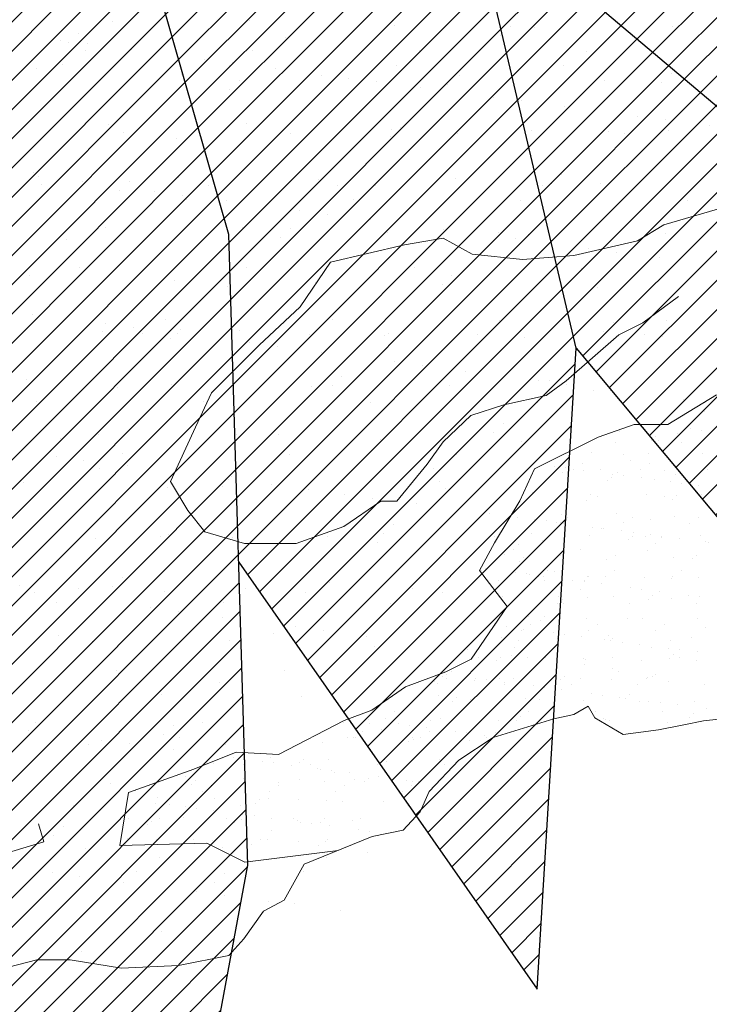
# Model space of a CAD drawing. Units: inches. Extents: x 1986 to 21484, y -1816 to 2016.
# Tile 26 of 85: x 2172.013 to 2177.15, y 1869.056 to 1876.389. Entities that reach past the tile are written whole.
import ezdxf

# ---------------------------------------------------------------- set-up
doc = ezdxf.new("R2010")
doc.units = ezdxf.units.IN
doc.layers.add('L-PLNT', color=84, linetype='Continuous', lineweight=13)
doc.layers.add('vfolhas', color=114, linetype='Continuous', lineweight=5)
for name, color, linetype in [('vfolha', 72, 'Continuous'), ('vfolha2', 110, 'Continuous'), ('vfolhas2', 102, 'Continuous')]:
    doc.layers.add(name, color=color, linetype=linetype)
pattern_1 = [(45, (-2446.5133113, 50.986076), (-0.004419417382, 0.004419417382), [])]

# ---------------------------------------------------------------- blocks, each defined once
blk = doc.blocks.new('arbusto_PB_verde_grande')
at = {"layer": 'vfolha2'}
h = blk.add_hatch(dxfattribs=at)
h.set_pattern_fill('ANSI31', color=256, scale=0.05, style=0)
h.set_pattern_definition(pattern_1)
h.paths.add_polyline_path([(-0.18963, 0.29704), (-0.08553, 0.20192), (-0.10785, 0.25007), (-0.13202, 0.31865), (-0.25096, 0.48479), (-0.44952, 0.5505), (-0.37946, 0.43789)])
h.paths.add_polyline_path([(0.07911, -0.4071), (0.08214, -0.50631), (0.17255, -0.6355), (0.18428, -0.44151), (0.14904, -0.29177), (0.02625, -0.03934), (0.03527, -0.25376)])
at = {"layer": 'vfolhas'}
h = blk.add_hatch(dxfattribs=at)
h.set_pattern_fill('ANSI31', color=256, scale=0.05, style=0)
h.set_pattern_definition(pattern_1)
h.paths.add_polyline_path([(-0.07279, 0.50669), (-0.18085, 0.65063), (-0.2334, 0.67253), (-0.20712, 0.53176), (-0.10785, 0.25007), (0.02625, -0.03934), (0.00028, 0.09048), (0.00816, 0.16241), (-0.04939, 0.29079)])
h.paths.add_polyline_path([(0.09902, 0.41929), (0.09372, 0.26573), (0.07906, 0.18814), (0.15506, 0.36901), (0.26606, 0.5505), (0.28356, 0.63504), (0.2485, 0.68819), (0.25145, 0.63504), (0.20178, 0.54426)])
h.paths.add_polyline_path([(0.12295, 0.24073), (0.047, 0.06233), (0.02625, -0.03934), (0.11122, 0.04358), (0.18428, 0.09364), (0.27478, 0.19376), (0.3215, 0.25323), (0.44129, 0.38467), (0.47634, 0.57866), (0.41789, 0.45347), (0.28939, 0.30954)])
h.paths.add_polyline_path([(0.58145, -0.03779), (0.70707, 0.01536), (0.78591, 0.04667), (0.74796, 0.06549), (0.62818, 0.08423), (0.52595, 0.09048), (0.39745, 0.04358), (0.02625, -0.03934), (0.25728, -0.03154), (0.43834, -0.0347)])
h.paths.add_polyline_path([(0.52022, -0.03647), (0.43834, -0.0347), (0.25728, -0.03154), (0.02625, -0.03934), (0.17964, -0.08515), (0.53768, -0.13167), (0.69541, -0.15357), (0.78591, -0.07852), (0.70413, -0.10042)])
h.paths.add_polyline_path([(0.27189, -0.21929), (0.14922, -0.14107), (0.02625, -0.03934), (0.15794, -0.31007), (0.29522, -0.42585), (0.41789, -0.49157), (0.56396, -0.56669), (0.5114, -0.48532), (0.39456, -0.34139)])
h.paths.add_polyline_path([(-0.05818, -0.47591), (-0.02312, -0.61984), (0.047, -0.80134), (0.08494, -0.59794), (0.07911, -0.4071), (0.03527, -0.25376), (0.02625, -0.03934), (-0.03773, -0.26001)])
h.paths.add_polyline_path([(-0.24218, 0.14054), (-0.11073, 0.06858), (0.02625, -0.03934), (-0.04235, 0.10871), (-0.21007, 0.23757), (-0.36485, 0.33145), (-0.47874, 0.40341), (-0.54303, 0.46288), (-0.49041, 0.33145), (-0.39408, 0.22192)])
h = blk.add_hatch(dxfattribs=at)
h.set_pattern_fill('ANSI31', color=256, scale=0.05, style=0)
h.set_pattern_definition(pattern_1)
h.paths.add_polyline_path([(0.33611, -0.623), (0.43251, -0.67306), (0.39456, -0.59485), (0.3303, -0.44464), (0.29522, -0.42585), (0.15794, -0.31007), (0.14904, -0.29177), (0.18428, -0.44151)])
at = {"layer": 'vfolha'}
for p, q in [((0.07911, -0.4071), (0.03527, -0.25376)), ((0.15794, -0.31007), (0.29522, -0.42585)), ((0.08494, -0.59794), (0.07911, -0.4071)), ((0.047, -0.80134), (0.08494, -0.59794))]:
    blk.add_line(p, q, dxfattribs=at)
at = {"layer": 'vfolha2'}
for p, q in [((0.18428, -0.44151), (0.14904, -0.29177)), ((0.17255, -0.6355), (0.18428, -0.44151)), ((0.08214, -0.50631), (0.17255, -0.6355))]:
    blk.add_line(p, q, dxfattribs=at)
at = {"layer": 'vfolhas2'}
blk.add_line((0.18428, -0.44151), (0.33611, -0.623), dxfattribs=at)
blk = doc.blocks.new('PLANT-SHRUB')
for p, q in [((2172.703, 1876.3791), (2172.703, 1876.3791)), ((2173.7254, 1876.384), (2173.7254, 1876.384)), ((2172.4474, 1876.2879), (2172.4474, 1876.2879)), ((2174.8049, 1876.3451), (2174.8049, 1876.3451)), ((2175.6695, 1876.3369), (2175.6695, 1876.3369)), ((2175.8511, 1876.3317), (2175.8511, 1876.3317)), ((2176.8734, 1876.3366), (2176.8734, 1876.3366)), ((2172.3132, 1876.2377), (2172.3132, 1876.2377)), ((2172.3737, 1876.2204), (2172.3737, 1876.2204)), ((2172.5213, 1876.2103), (2172.5213, 1876.2103)), ((2173.9965, 1876.2557), (2173.9965, 1876.2557)), ((2175.5958, 1876.2694), (2175.5958, 1876.2694)), ((2172.5, 1876.1609), (2172.5, 1876.1609)), ((2172.8462, 1876.1675), (2172.8462, 1876.1675)), ((2173.7446, 1876.1587), (2173.7446, 1876.1587)), ((2174.9892, 1876.1564), (2174.9892, 1876.1564)), ((2176.2339, 1876.1542), (2176.2339, 1876.1542)), ((2173.3891, 1876.096), (2173.3891, 1876.096)), ((2173.5971, 1876.0686), (2173.5971, 1876.0686)), ((2172.1388, 1876.0226), (2172.1388, 1876.0226)), ((2172.3314, 1876.0536), (2172.3314, 1876.0536)), ((2173.2183, 1875.9837), (2173.2183, 1875.9837)), ((2173.576, 1876.0513), (2173.576, 1876.0513)), ((2173.922, 1876.0259), (2173.922, 1876.0259)), ((2174.8207, 1876.049), (2174.8207, 1876.049)), ((2176.0653, 1876.0468), (2176.0653, 1876.0468)), ((2176.8709, 1875.9862), (2176.8709, 1875.9862)), ((2173.6488, 1875.9371), (2173.6488, 1875.9371)), ((2174.2644, 1875.9703), (2174.2644, 1875.9703)), ((2174.4649, 1875.9544), (2174.4649, 1875.9544)), ((2174.6729, 1875.927), (2174.6729, 1875.927)), ((2175.2868, 1875.9752), (2175.2868, 1875.9752)), ((2176.3663, 1875.9364), (2176.3663, 1875.9364)), ((2176.7973, 1875.9187), (2176.7973, 1875.9187)), ((2173.5752, 1875.8696), (2173.5752, 1875.8696)), ((2174.9978, 1875.8842), (2174.9978, 1875.8842)), ((2175.198, 1875.9049), (2175.198, 1875.9049)), ((2175.5407, 1875.8127), (2175.5407, 1875.8127)), ((2175.7487, 1875.7854), (2175.7487, 1875.7854)), ((2176.0737, 1875.7426), (2176.0737, 1875.7426)), ((2176.6165, 1875.6711), (2176.6165, 1875.6711)), ((2176.8246, 1875.6437), (2176.8246, 1875.6437)), ((2172.6778, 1875.609), (2172.6778, 1875.609)), ((2172.7839, 1875.5467), (2172.7839, 1875.5467)), ((2173.7002, 1875.6139), (2173.7002, 1875.6139)), ((2174.0285, 1875.5444), (2174.0285, 1875.5444)), ((2174.7797, 1875.575), (2174.7797, 1875.575)), ((2174.8503, 1875.5863), (2174.8503, 1875.5863)), ((2175.2732, 1875.5421), (2175.2732, 1875.5421)), ((2175.8259, 1875.5616), (2175.8259, 1875.5616)), ((2176.3995, 1875.5541), (2176.3995, 1875.5541)), ((2176.8483, 1875.5665), (2176.8483, 1875.5665)), ((2177.1495, 1875.6009), (2177.1495, 1875.6009)), ((2173.1774, 1875.5051), (2173.1774, 1875.5051)), ((2174.7766, 1875.5188), (2174.7766, 1875.5188)), ((2176.5178, 1875.5399), (2176.5178, 1875.5399)), ((2172.1136, 1875.2525), (2172.1136, 1875.2525)), ((2172.1528, 1875.224), (2172.1528, 1875.224)), ((2172.4777, 1875.1812), (2172.4777, 1875.1812)), ((2172.8296, 1875.1865), (2172.8296, 1875.1865)), ((2173.1931, 1875.2136), (2173.1931, 1875.2136)), ((2174.2393, 1875.2002), (2174.2393, 1875.2002)), ((2175.2617, 1875.2051), (2175.2617, 1875.2051)), ((2176.0518, 1875.2355), (2176.0518, 1875.2355)), ((2172.1772, 1875.1601), (2172.1772, 1875.1601)), ((2172.756, 1875.119), (2172.756, 1875.119)), ((2173.0206, 1875.1097), (2173.0206, 1875.1097)), ((2173.4218, 1875.1579), (2173.4218, 1875.1579)), ((2174.3788, 1875.1543), (2174.3788, 1875.1543)), ((2174.6664, 1875.1556), (2174.6664, 1875.1556)), ((2175.9111, 1875.1533), (2175.9111, 1875.1533)), ((2175.9781, 1875.168), (2175.9781, 1875.168)), ((2176.3411, 1875.1663), (2176.3411, 1875.1663)), ((2173.2286, 1875.0823), (2173.2286, 1875.0823)), ((2173.2533, 1875.0505), (2173.2533, 1875.0505)), ((2173.5535, 1875.0396), (2173.5535, 1875.0396)), ((2174.4979, 1875.0482), (2174.4979, 1875.0482)), ((2175.7425, 1875.046), (2175.7425, 1875.046)), ((2177.5527, 1875.0804), (2176.8121, 1874.8603)), ((2176.9872, 1875.0437), (2176.9872, 1875.0437)), ((2174.0964, 1874.9681), (2174.0964, 1874.9681)), ((2174.3044, 1874.9407), (2174.3044, 1874.9407)), ((2174.6293, 1874.8979), (2174.6293, 1874.8979)), ((2172.6527, 1874.8389), (2172.6527, 1874.8389)), ((2173.6751, 1874.8438), (2173.6751, 1874.8438)), ((2174.0311, 1874.8357), (2174.0311, 1874.8357)), ((2175.1722, 1874.8265), (2175.1722, 1874.8265)), ((2176.8121, 1874.8603), (2176.6151, 1874.7421)), ((2172.3582, 1874.7544), (2172.3582, 1874.7544)), ((2173.9574, 1874.7682), (2173.9574, 1874.7682)), ((2174.7545, 1874.8049), (2174.7545, 1874.8049)), ((2175.1665, 1874.7618), (2174.8807, 1874.7126)), ((2175.3833, 1874.6437), (2175.1665, 1874.7618)), ((2175.3802, 1874.7991), (2175.3802, 1874.7991)), ((2175.5803, 1874.8035), (2175.5803, 1874.8035)), ((2175.7052, 1874.7563), (2175.7052, 1874.7563)), ((2175.8007, 1874.7915), (2175.8007, 1874.7915)), ((2176.6151, 1874.7421), (2176.142, 1874.6338)), ((2176.8231, 1874.7964), (2176.8231, 1874.7964)), ((2174.8807, 1874.7126), (2174.3288, 1874.5846)), ((2176.248, 1874.6848), (2176.248, 1874.6848)), ((2175.7577, 1874.6043), (2175.3833, 1874.6437)), ((2176.142, 1874.6338), (2175.7577, 1874.6043)), ((2176.4561, 1874.6574), (2176.4561, 1874.6574)), ((2176.781, 1874.6147), (2176.781, 1874.6147)), ((2172.4611, 1874.5458), (2172.4611, 1874.5458)), ((2173.7058, 1874.5436), (2173.7058, 1874.5436)), ((2174.3288, 1874.5846), (2174.1022, 1874.2498)), ((2174.9504, 1874.5413), (2174.9504, 1874.5413)), ((2176.195, 1874.5391), (2176.195, 1874.5391)), ((2172.0884, 1874.4824), (2172.0884, 1874.4824)), ((2173.1679, 1874.4435), (2173.1679, 1874.4435)), ((2175.2326, 1874.4849), (2175.2326, 1874.4849)), ((2176.7817, 1874.4527), (2176.7817, 1874.4527)), ((2173.5596, 1874.4037), (2173.5596, 1874.4037)), ((2174.2141, 1874.4301), (2174.2141, 1874.4301)), ((2175.1589, 1874.4174), (2175.1589, 1874.4174)), ((2175.2365, 1874.4351), (2175.2365, 1874.4351)), ((2176.316, 1874.3962), (2176.316, 1874.3962)), ((2176.6545, 1874.1316), (2176.9205, 1874.3286)), ((2176.9205, 1874.3286), (2176.9205, 1874.3286)), ((2174.1022, 1874.2498), (2173.7967, 1873.9642)), ((2174.1022, 1874.2498), (2174.1022, 1874.2498)), ((2172.1092, 1874.1949), (2172.1092, 1874.1949)), ((2173.099, 1874.157), (2173.099, 1874.157)), ((2174.3436, 1874.1548), (2174.3436, 1874.1548)), ((2175.5883, 1874.1525), (2175.5883, 1874.1525)), ((2176.8329, 1874.1503), (2176.8329, 1874.1503)), ((2172.6521, 1874.1234), (2172.6521, 1874.1234)), ((2172.8601, 1874.096), (2172.8601, 1874.096)), ((2173.2119, 1874.085), (2173.2119, 1874.085)), ((2176.434, 1874.1341), (2176.434, 1874.1341)), ((2176.4771, 1874.043), (2176.6545, 1874.1316)), ((2172.6275, 1874.0688), (2172.6275, 1874.0688)), ((2172.9305, 1874.0497), (2172.9305, 1874.0497)), ((2173.1383, 1874.0175), (2173.1383, 1874.0175)), ((2173.185, 1874.0533), (2173.185, 1874.0533)), ((2173.6499, 1874.0737), (2173.6499, 1874.0737)), ((2174.1751, 1874.0474), (2174.1751, 1874.0474)), ((2174.7293, 1874.0348), (2174.7293, 1874.0348)), ((2174.7611, 1874.0529), (2174.7611, 1874.0529)), ((2175.4197, 1874.0451), (2175.4197, 1874.0451)), ((2175.7755, 1874.0214), (2175.7755, 1874.0214)), ((2176.0829, 1873.6984), (2176.4771, 1874.043)), ((2176.3604, 1874.0666), (2176.3604, 1874.0666)), ((2176.6644, 1874.0429), (2176.6644, 1874.0429)), ((2176.7979, 1874.0263), (2176.7979, 1874.0263)), ((2173.7967, 1873.9642), (2173.4419, 1873.6097)), ((2173.7279, 1873.9818), (2173.7279, 1873.9818)), ((2173.9359, 1873.9544), (2173.9359, 1873.9544)), ((2174.2608, 1873.9116), (2174.2608, 1873.9116)), ((2174.8037, 1873.8402), (2174.8037, 1873.8402)), ((2175.0117, 1873.8128), (2175.0117, 1873.8128)), ((2172.0633, 1873.7123), (2172.0633, 1873.7123)), ((2174.4134, 1873.7343), (2174.4134, 1873.7343)), ((2175.3367, 1873.77), (2175.3367, 1873.77)), ((2172.7405, 1873.653), (2172.7405, 1873.653)), ((2173.1427, 1873.6734), (2173.1427, 1873.6734)), ((2174.1889, 1873.6601), (2174.1889, 1873.6601)), ((2174.3397, 1873.6667), (2174.3397, 1873.6667)), ((2175.2113, 1873.665), (2175.2113, 1873.665)), ((2175.8795, 1873.6985), (2175.8795, 1873.6985)), ((2175.9351, 1873.5901), (2176.0829, 1873.6984)), ((2175.9626, 1873.7021), (2175.9626, 1873.7021)), ((2176.0876, 1873.6711), (2176.0876, 1873.6711)), ((2173.4419, 1873.6097), (2173.3237, 1873.3537)), ((2175.6198, 1873.5211), (2175.9351, 1873.5901)), ((2176.2908, 1873.6261), (2176.2908, 1873.6261)), ((2176.4125, 1873.6284), (2176.4125, 1873.6284)), ((2177.2044, 1873.5947), (2176.8418, 1873.3742)), ((2172.1383, 1873.545), (2172.1383, 1873.545)), ((2173.383, 1873.5428), (2173.383, 1873.5428)), ((2174.6276, 1873.5405), (2174.6276, 1873.5405)), ((2175.3734, 1873.4424), (2175.6198, 1873.5211)), ((2175.8722, 1873.5382), (2175.8722, 1873.5382)), ((2176.9554, 1873.5569), (2176.9554, 1873.5569)), ((2177.1169, 1873.536), (2177.1169, 1873.536)), ((2175.1665, 1873.2454), (2175.3734, 1873.4424)), ((2177.1132, 1873.4687), (2177.1132, 1873.4687)), ((2173.3237, 1873.3537), (2173.1364, 1872.95)), ((2175.6149, 1873.3835), (2175.6149, 1873.3835)), ((2176.5897, 1873.3742), (2176.3217, 1873.2797)), ((2176.8418, 1873.3742), (2176.5897, 1873.3742)), ((2176.7893, 1873.3718), (2176.7893, 1873.3718)), ((2176.8418, 1873.3742), (2176.8418, 1873.3742)), ((2177.0065, 1873.3432), (2177.0065, 1873.3432)), ((2172.3928, 1873.3344), (2172.3928, 1873.3344)), ((2172.6023, 1873.2987), (2172.6023, 1873.2987)), ((2173.6247, 1873.3036), (2173.6247, 1873.3036)), ((2173.9419, 1873.3022), (2173.9419, 1873.3022)), ((2175.5412, 1873.316), (2175.5412, 1873.316)), ((2176.3217, 1873.2797), (2175.8488, 1873.0435)), ((2176.4785, 1873.3241), (2176.4785, 1873.3241)), ((2176.7503, 1873.2826), (2176.7503, 1873.2826)), ((2176.9103, 1873.3086), (2176.9103, 1873.3086)), ((2177.0897, 1873.3322), (2177.0897, 1873.3322)), ((2172.3191, 1873.2669), (2172.3191, 1873.2669)), ((2174.7042, 1873.2647), (2174.7042, 1873.2647)), ((2175.0482, 1873.078), (2175.1665, 1873.2454)), ((2175.1665, 1873.2454), (2175.1665, 1873.2454)), ((2175.7503, 1873.2513), (2175.7503, 1873.2513)), ((2176.4488, 1873.2405), (2176.4488, 1873.2405)), ((2176.7209, 1873.2556), (2176.7209, 1873.2556)), ((2176.7727, 1873.2562), (2176.7727, 1873.2562)), ((2176.9467, 1873.2396), (2176.9467, 1873.2396)), ((2172.2836, 1873.1371), (2172.2836, 1873.1371)), ((2172.7762, 1873.1562), (2172.7762, 1873.1562)), ((2174.0209, 1873.154), (2174.0209, 1873.154)), ((2175.2655, 1873.1517), (2175.2655, 1873.1517)), ((2176.2757, 1873.164), (2176.2757, 1873.164)), ((2176.5101, 1873.1494), (2176.5101, 1873.1494)), ((2176.6941, 1873.1587), (2176.6941, 1873.1587)), ((2177.1031, 1873.1606), (2177.1031, 1873.1606)), ((2172.4916, 1873.1097), (2172.4916, 1873.1097)), ((2172.6077, 1873.0489), (2172.6077, 1873.0489)), ((2172.8165, 1873.067), (2172.8165, 1873.067)), ((2174.8216, 1872.8023), (2175.0482, 1873.078)), ((2175.9984, 1873.062), (2175.9984, 1873.062)), ((2176.0816, 1873.051), (2176.0816, 1873.051)), ((2176.2061, 1873.0859), (2176.2061, 1873.0859)), ((2176.5617, 1873.1098), (2176.5617, 1873.1098)), ((2176.704, 1873.085), (2176.704, 1873.085)), ((2173.3594, 1872.9955), (2173.3594, 1872.9955)), ((2173.5942, 1872.9836), (2173.5942, 1872.9836)), ((2173.8523, 1873.0466), (2173.8523, 1873.0466)), ((2175.097, 1873.0443), (2175.097, 1873.0443)), ((2175.8488, 1873.0435), (2175.7385, 1872.8072)), ((2176.0595, 1873.0141), (2176.0595, 1873.0141)), ((2176.1387, 1873.043), (2176.1387, 1873.043)), ((2176.2116, 1873.0339), (2176.2116, 1873.0339)), ((2176.3416, 1873.0421), (2176.3416, 1873.0421)), ((2176.4227, 1872.9824), (2176.4227, 1872.9824)), ((2176.4288, 1873.0053), (2176.4288, 1873.0053)), ((2176.4685, 1873.0161), (2176.4685, 1873.0161)), ((2176.512, 1872.9944), (2176.512, 1872.9944)), ((2176.6365, 1873.0421), (2176.6365, 1873.0421)), ((2176.6419, 1872.9773), (2176.6419, 1872.9773)), ((2176.8163, 1873.0327), (2176.8163, 1873.0327)), ((2176.9002, 1873.0005), (2176.9002, 1873.0005)), ((2177.1344, 1873.0412), (2177.1344, 1873.0412)), ((2172.0381, 1872.9422), (2172.0381, 1872.9422)), ((2173.1176, 1872.9033), (2173.1176, 1872.9033)), ((2173.1364, 1872.95), (2173.2646, 1872.7334)), ((2173.5205, 1872.9161), (2173.5205, 1872.9161)), ((2173.5674, 1872.9681), (2173.5674, 1872.9681)), ((2173.8924, 1872.9253), (2173.8924, 1872.9253)), ((2175.1434, 1872.9514), (2175.1434, 1872.9514)), ((2176.3932, 1872.9554), (2176.3932, 1872.9554)), ((2176.7427, 1872.9652), (2176.7427, 1872.9652)), ((2176.8591, 1872.9487), (2176.8591, 1872.9487)), ((2176.9423, 1872.9377), (2176.9423, 1872.9377)), ((2177.0423, 1872.9695), (2177.0423, 1872.9695)), ((2177.0723, 1872.9206), (2177.0723, 1872.9206)), ((2174.1637, 1872.89), (2174.1637, 1872.89)), ((2174.4352, 1872.8539), (2174.4352, 1872.8539)), ((2175.1861, 1872.8949), (2175.1861, 1872.8949)), ((2175.8218, 1872.8411), (2175.8218, 1872.8411)), ((2175.8338, 1872.8715), (2175.8338, 1872.8715)), ((2176.2656, 1872.856), (2176.2656, 1872.856)), ((2176.2656, 1872.856), (2176.2656, 1872.856)), ((2176.3197, 1872.8402), (2176.3197, 1872.8402)), ((2176.6841, 1872.8506), (2176.6841, 1872.8506)), ((2176.8175, 1872.8393), (2176.8175, 1872.8393)), ((2176.9032, 1872.8421), (2176.9032, 1872.8421)), ((2177.093, 1872.8526), (2177.093, 1872.8526)), ((2174.4274, 1872.6152), (2174.7033, 1872.8023)), ((2174.6433, 1872.8265), (2174.6433, 1872.8265)), ((2174.7033, 1872.8023), (2174.8216, 1872.8023)), ((2174.9682, 1872.7837), (2174.9682, 1872.7837)), ((2175.7385, 1872.8072), (2175.5494, 1872.4923)), ((2176.2341, 1872.8096), (2176.2341, 1872.8096)), ((2176.8738, 1872.8151), (2176.8738, 1872.8151)), ((2173.2646, 1872.7334), (2173.3927, 1872.5758)), ((2175.511, 1872.7122), (2175.511, 1872.7122)), ((2175.7191, 1872.6848), (2175.7191, 1872.6848)), ((2176.0494, 1872.7061), (2176.0494, 1872.7061)), ((2176.077, 1872.6856), (2176.077, 1872.6856)), ((2176.095, 1872.6821), (2176.095, 1872.6821)), ((2176.4584, 1872.708), (2176.4584, 1872.708)), ((2176.5748, 1872.6847), (2176.5748, 1872.6847)), ((2176.8902, 1872.6925), (2176.8902, 1872.6925)), ((2177.0727, 1872.6838), (2177.0727, 1872.6838)), ((2174.0726, 1872.4872), (2174.4274, 1872.6152)), ((2174.7957, 1872.6328), (2174.7957, 1872.6328)), ((2175.851, 1872.6675), (2175.851, 1872.6675)), ((2175.9342, 1872.6565), (2175.9342, 1872.6565)), ((2176.0096, 1872.6426), (2176.0096, 1872.6426)), ((2176.044, 1872.6421), (2176.044, 1872.6421)), ((2176.0642, 1872.6394), (2176.0642, 1872.6394)), ((2176.0655, 1872.6551), (2176.0655, 1872.6551)), ((2176.2814, 1872.6108), (2176.2814, 1872.6108)), ((2176.5074, 1872.6417), (2176.5074, 1872.6417)), ((2176.7147, 1872.6693), (2176.7147, 1872.6693)), ((2177.0053, 1872.6408), (2177.0053, 1872.6408)), ((2173.0602, 1872.5419), (2173.0602, 1872.5419)), ((2173.1227, 1872.5516), (2173.1227, 1872.5516)), ((2173.3927, 1872.5758), (2173.6883, 1872.4872)), ((2174.3048, 1872.5397), (2174.3048, 1872.5397)), ((2174.722, 1872.5653), (2174.722, 1872.5653)), ((2175.5495, 1872.5374), (2175.5495, 1872.5374)), ((2175.8237, 1872.5635), (2175.8237, 1872.5635)), ((2176.2555, 1872.5479), (2176.2555, 1872.5479)), ((2176.3448, 1872.6007), (2176.3448, 1872.6007)), ((2176.3646, 1872.5999), (2176.3646, 1872.5999)), ((2176.4945, 1872.5827), (2176.4945, 1872.5827)), ((2176.5756, 1872.5418), (2176.5756, 1872.5418)), ((2176.5869, 1872.5706), (2176.5869, 1872.5706)), ((2176.674, 1872.5426), (2176.674, 1872.5426)), ((2176.7117, 1872.5542), (2176.7117, 1872.5542)), ((2176.7941, 1872.5352), (2176.7941, 1872.5352)), ((2176.7949, 1872.5432), (2176.7949, 1872.5432)), ((2176.7949, 1872.5432), (2176.7949, 1872.5432)), ((2177.083, 1872.5446), (2177.083, 1872.5446)), ((2172.5771, 1872.5286), (2172.5771, 1872.5286)), ((2173.5995, 1872.5335), (2173.5995, 1872.5335)), ((2173.6883, 1872.4872), (2173.9149, 1872.4872)), ((2173.9149, 1872.4872), (2174.0726, 1872.4872)), ((2174.679, 1872.4946), (2174.679, 1872.4946)), ((2175.5494, 1872.4923), (2175.439, 1872.2875)), ((2175.7252, 1872.4812), (2175.7252, 1872.4812)), ((2175.9064, 1872.5093), (2175.9064, 1872.5093)), ((2176.5461, 1872.5148), (2176.5461, 1872.5148)), ((2176.7476, 1872.4861), (2176.7476, 1872.4861)), ((2176.9249, 1872.5261), (2176.9249, 1872.5261)), ((2177.1198, 1872.5004), (2177.1198, 1872.5004)), ((2177.142, 1872.4975), (2177.142, 1872.4975)), ((2175.6209, 1872.4034), (2175.6209, 1872.4034)), ((2175.6927, 1872.4408), (2175.6927, 1872.4408)), ((2176.0394, 1872.398), (2176.0394, 1872.398)), ((2176.1906, 1872.4399), (2176.1906, 1872.4399)), ((2176.4483, 1872.4), (2176.4483, 1872.4)), ((2176.6884, 1872.439), (2176.6884, 1872.439)), ((2177.0562, 1872.4015), (2177.0562, 1872.4015)), ((2175.7378, 1872.3549), (2175.7378, 1872.3549)), ((2175.7673, 1872.3819), (2175.7673, 1872.3819)), ((2176.387, 1872.369), (2176.387, 1872.369)), ((2176.8801, 1872.3844), (2176.8801, 1872.3844)), ((2177.0267, 1872.3745), (2177.0267, 1872.3745)), ((2175.439, 1872.2875), (2175.6439, 1872.0198)), ((2175.45, 1872.2862), (2175.45, 1872.2862)), ((2175.4865, 1872.3015), (2175.4865, 1872.3015)), ((2175.7036, 1872.2729), (2175.7036, 1872.2729)), ((2175.7868, 1872.262), (2175.7868, 1872.262)), ((2175.8137, 1872.2554), (2175.8137, 1872.2554)), ((2175.8805, 1872.2423), (2175.8805, 1872.2423)), ((2175.9168, 1872.2449), (2175.9168, 1872.2449)), ((2175.9479, 1872.2853), (2175.9479, 1872.2853)), ((2175.9971, 1872.2821), (2175.9971, 1872.2821)), ((2176.2479, 1872.2416), (2176.2479, 1872.2416)), ((2176.3783, 1872.2414), (2176.3783, 1872.2414)), ((2176.4457, 1872.2844), (2176.4457, 1872.2844)), ((2176.9436, 1872.2835), (2176.9436, 1872.2835)), ((2172.0129, 1872.1721), (2172.0129, 1872.1721)), ((2172.775, 1872.233), (2172.775, 1872.233)), ((2174.3242, 1872.2008), (2174.3242, 1872.2008)), ((2175.5787, 1872.2091), (2175.5787, 1872.2091)), ((2175.9235, 1872.2145), (2175.9235, 1872.2145)), ((2176.134, 1872.2163), (2176.134, 1872.2163)), ((2176.2172, 1872.2053), (2176.2172, 1872.2053)), ((2176.2184, 1872.2145), (2176.2184, 1872.2145)), ((2176.2455, 1872.2399), (2176.2455, 1872.2399)), ((2176.3471, 1872.1882), (2176.3471, 1872.1882)), ((2176.6639, 1872.2346), (2176.6639, 1872.2346)), ((2176.8676, 1872.2287), (2176.8676, 1872.2287)), ((2176.8762, 1872.2405), (2176.8762, 1872.2405)), ((2177.0729, 1872.2365), (2177.0729, 1872.2365)), ((2172.1231, 1872.1234), (2172.1231, 1872.1234)), ((2172.4534, 1872.1554), (2172.4534, 1872.1554)), ((2172.7014, 1872.1655), (2172.7014, 1872.1655)), ((2173.0924, 1872.1332), (2173.0924, 1872.1332)), ((2173.6981, 1872.1531), (2173.6981, 1872.1531)), ((2174.1386, 1872.1199), (2174.1386, 1872.1199)), ((2174.9427, 1872.1509), (2174.9427, 1872.1509)), ((2175.161, 1872.1248), (2175.161, 1872.1248)), ((2175.6108, 1872.0953), (2175.6108, 1872.0953)), ((2176.1873, 1872.1486), (2176.1873, 1872.1486)), ((2176.5643, 1872.1596), (2176.5643, 1872.1596)), ((2176.6475, 1872.1487), (2176.6475, 1872.1487)), ((2176.7285, 1872.1012), (2176.7285, 1872.1012)), ((2176.7775, 1872.1316), (2176.7775, 1872.1316)), ((2176.9946, 1872.103), (2176.9946, 1872.103)), ((2172.2849, 1872.048), (2172.2849, 1872.048)), ((2172.448, 1872.0807), (2172.448, 1872.0807)), ((2173.5295, 1872.0458), (2173.5295, 1872.0458)), ((2174.7742, 1872.0435), (2174.7742, 1872.0435)), ((2176.0188, 1872.0413), (2176.0188, 1872.0413)), ((2176.0293, 1872.09), (2176.0293, 1872.09)), ((2176.0593, 1872.0687), (2176.0593, 1872.0687)), ((2176.0615, 1872.0396), (2176.0615, 1872.0396)), ((2176.2404, 1872.0859), (2176.2404, 1872.0859)), ((2176.4382, 1872.092), (2176.4382, 1872.092)), ((2176.5593, 1872.0387), (2176.5593, 1872.0387)), ((2176.699, 1872.0742), (2176.699, 1872.0742)), ((2176.87, 1872.0764), (2176.87, 1872.0764)), ((2177.0572, 1872.0377), (2177.0572, 1872.0377)), ((2177.0778, 1872.092), (2177.0778, 1872.092)), ((2172.9909, 1872.0092), (2172.9909, 1872.0092)), ((2173.1989, 1871.9818), (2173.1989, 1871.9818)), ((2175.6439, 1872.0198), (2175.376, 1871.626)), ((2173.5239, 1871.939), (2173.5239, 1871.939)), ((2173.9765, 1871.8822), (2173.9765, 1871.8822)), ((2175.5562, 1871.8784), (2175.5562, 1871.8784)), ((2175.8036, 1871.9474), (2175.8036, 1871.9474)), ((2175.8188, 1871.8849), (2175.8188, 1871.8849)), ((2175.8908, 1871.9143), (2175.8908, 1871.9143)), ((2175.9202, 1871.9413), (2175.9202, 1871.9413)), ((2176.2354, 1871.9319), (2176.2354, 1871.9319)), ((2176.3166, 1871.884), (2176.3166, 1871.884)), ((2176.5399, 1871.9284), (2176.5399, 1871.9284)), ((2176.6539, 1871.9265), (2176.6539, 1871.9265)), ((2176.8145, 1871.8831), (2176.8145, 1871.8831)), ((2177.0628, 1871.9285), (2177.0628, 1871.9285)), ((2173.9028, 1871.8147), (2173.9028, 1871.8147)), ((2174.0667, 1871.8676), (2174.0667, 1871.8676)), ((2174.2748, 1871.8402), (2174.2748, 1871.8402)), ((2175.5257, 1871.85), (2175.5257, 1871.85)), ((2175.6394, 1871.8675), (2175.6394, 1871.8675)), ((2175.7514, 1871.842), (2175.7514, 1871.842)), ((2175.7694, 1871.8504), (2175.7694, 1871.8504)), ((2175.9866, 1871.8218), (2175.9866, 1871.8218)), ((2176.0698, 1871.8108), (2176.0698, 1871.8108)), ((2176.2492, 1871.8411), (2176.2492, 1871.8411)), ((2176.7471, 1871.8402), (2176.7471, 1871.8402)), ((2177.1249, 1871.8638), (2177.1249, 1871.8638)), ((2172.3036, 1871.801), (2172.3036, 1871.801)), ((2172.552, 1871.7585), (2172.552, 1871.7585)), ((2173.5743, 1871.7634), (2173.5743, 1871.7634)), ((2174.5997, 1871.7974), (2174.5997, 1871.7974)), ((2175.6007, 1871.7873), (2175.6007, 1871.7873)), ((2175.7316, 1871.7685), (2175.7316, 1871.7685)), ((2176.0192, 1871.782), (2176.0192, 1871.782)), ((2176.1997, 1871.7937), (2176.1997, 1871.7937)), ((2176.3713, 1871.774), (2176.3713, 1871.774)), ((2176.4008, 1871.801), (2176.4008, 1871.801)), ((2176.4169, 1871.7651), (2176.4169, 1871.7651)), ((2176.4282, 1871.7839), (2176.4282, 1871.7839)), ((2176.5001, 1871.7542), (2176.5001, 1871.7542)), ((2176.6301, 1871.7371), (2176.6301, 1871.7371)), ((2176.86, 1871.7684), (2176.86, 1871.7684)), ((2177.0205, 1871.7881), (2177.0205, 1871.7881)), ((2174.6538, 1871.7245), (2174.6538, 1871.7245)), ((2175.1425, 1871.7259), (2175.1425, 1871.7259)), ((2175.3506, 1871.6985), (2175.3506, 1871.6985)), ((2175.6755, 1871.6558), (2175.6755, 1871.6558)), ((2175.7, 1871.7111), (2175.7, 1871.7111)), ((2176.7224, 1871.7161), (2176.7224, 1871.7161)), ((2176.8472, 1871.7085), (2176.8472, 1871.7085)), ((2176.8814, 1871.6607), (2176.8814, 1871.6607)), ((2176.9304, 1871.6975), (2176.9304, 1871.6975)), ((2177.0604, 1871.6804), (2177.0604, 1871.6804)), ((2175.376, 1871.626), (2175.1869, 1871.5315)), ((2175.3846, 1871.6374), (2175.3846, 1871.6374)), ((2175.4345, 1871.6401), (2175.4345, 1871.6401)), ((2175.5631, 1871.614), (2175.5631, 1871.614)), ((2175.5926, 1871.641), (2175.5926, 1871.641)), ((2175.7935, 1871.6394), (2175.7935, 1871.6394)), ((2175.9323, 1871.6392), (2175.9323, 1871.6392)), ((2176.2122, 1871.6282), (2176.2122, 1871.6282)), ((2176.2184, 1871.5843), (2176.2184, 1871.5843)), ((2176.2253, 1871.6238), (2176.2253, 1871.6238)), ((2176.4302, 1871.6383), (2176.4302, 1871.6383)), ((2176.6438, 1871.6185), (2176.6438, 1871.6185)), ((2176.8519, 1871.6337), (2176.8519, 1871.6337)), ((2176.9281, 1871.6374), (2176.9281, 1871.6374)), ((2177.0527, 1871.6204), (2177.0527, 1871.6204)), ((2172.7374, 1871.5411), (2172.7374, 1871.5411)), ((2173.982, 1871.5389), (2173.982, 1871.5389)), ((2175.1869, 1871.5315), (2174.8874, 1871.4213)), ((2175.178, 1871.5314), (2175.178, 1871.5314)), ((2175.1869, 1871.5315), (2175.1869, 1871.5315)), ((2175.1917, 1871.5125), (2175.1917, 1871.5125)), ((2175.2267, 1871.5366), (2175.2267, 1871.5366)), ((2176.4264, 1871.5569), (2176.4264, 1871.5569)), ((2176.4713, 1871.5343), (2176.4713, 1871.5343)), ((2176.7513, 1871.5141), (2176.7513, 1871.5141)), ((2173.505, 1871.4502), (2173.505, 1871.4502)), ((2175.1043, 1871.4639), (2175.1043, 1871.4639)), ((2175.1244, 1871.4426), (2175.1244, 1871.4426)), ((2175.1589, 1871.4948), (2175.1589, 1871.4948)), ((2175.1918, 1871.4855), (2175.1918, 1871.4855)), ((2175.404, 1871.4682), (2175.404, 1871.4682)), ((2175.4088, 1871.4839), (2175.4088, 1871.4839)), ((2175.492, 1871.473), (2175.492, 1871.473)), ((2175.5907, 1871.4793), (2175.5907, 1871.4793)), ((2175.622, 1871.4558), (2175.622, 1871.4558)), ((2175.6222, 1871.4417), (2175.6222, 1871.4417)), ((2175.6897, 1871.4846), (2175.6897, 1871.4846)), ((2176.0091, 1871.4739), (2176.0091, 1871.4739)), ((2176.0437, 1871.4737), (2176.0437, 1871.4737)), ((2176.0731, 1871.5007), (2176.0731, 1871.5007)), ((2176.1201, 1871.4408), (2176.1201, 1871.4408)), ((2176.1875, 1871.4837), (2176.1875, 1871.4837)), ((2176.4181, 1871.4759), (2176.4181, 1871.4759)), ((2176.6179, 1871.4399), (2176.6179, 1871.4399)), ((2176.6854, 1871.4828), (2176.6854, 1871.4828)), ((2176.6928, 1871.4879), (2176.6928, 1871.4879)), ((2176.7271, 1871.4992), (2176.7271, 1871.4992)), ((2176.8499, 1871.4603), (2176.8499, 1871.4603)), ((2177.1158, 1871.439), (2177.1158, 1871.439)), ((2173.0672, 1871.3631), (2173.0672, 1871.3631)), ((2174.8874, 1871.4213), (2174.6352, 1871.248)), ((2174.8874, 1871.4213), (2174.8874, 1871.4213)), ((2175.8392, 1871.4273), (2175.8392, 1871.4273)), ((2175.9224, 1871.4163), (2175.9224, 1871.4163)), ((2176.0523, 1871.3992), (2176.0523, 1871.3992)), ((2176.2695, 1871.3706), (2176.2695, 1871.3706)), ((2174.1134, 1871.3498), (2174.1134, 1871.3498)), ((2174.956, 1871.3347), (2174.956, 1871.3347)), ((2175.1358, 1871.3547), (2175.1358, 1871.3547)), ((2175.2354, 1871.3138), (2175.2354, 1871.3138)), ((2175.2649, 1871.3408), (2175.2649, 1871.3408)), ((2175.3745, 1871.3294), (2175.3745, 1871.3294)), ((2175.7835, 1871.3313), (2175.7835, 1871.3313)), ((2175.8846, 1871.3279), (2175.8846, 1871.3279)), ((2176.2152, 1871.3158), (2176.2152, 1871.3158)), ((2176.2152, 1871.3158), (2176.2152, 1871.3158)), ((2176.3527, 1871.3596), (2176.3527, 1871.3596)), ((2176.4827, 1871.3425), (2176.4827, 1871.3425)), ((2176.5243, 1871.3334), (2176.5243, 1871.3334)), ((2176.5537, 1871.3604), (2176.5537, 1871.3604)), ((2176.6337, 1871.3104), (2176.6337, 1871.3104)), ((2176.6998, 1871.3139), (2176.6998, 1871.3139)), ((2176.783, 1871.303), (2176.783, 1871.303)), ((2177.0427, 1871.3124), (2177.0427, 1871.3124)), ((2174.6352, 1871.248), (2174.4303, 1871.1693)), ((2174.8075, 1871.2407), (2174.8075, 1871.2407)), ((2175.3054, 1871.2398), (2175.3054, 1871.2398)), ((2175.8032, 1871.2389), (2175.8032, 1871.2389)), ((2176.1409, 1871.2146), (2175.9918, 1871.1818)), ((2176.247, 1871.2765), (2176.1409, 1871.2146)), ((2176.298, 1871.1891), (2176.247, 1871.2765)), ((2176.3011, 1871.238), (2176.3011, 1871.238)), ((2176.7989, 1871.2371), (2176.7989, 1871.2371)), ((2176.913, 1871.2859), (2176.913, 1871.2859)), ((2177.0343, 1871.2201), (2177.0343, 1871.2201)), ((2177.1302, 1871.2573), (2177.1302, 1871.2573)), ((2172.1307, 1871.1546), (2172.1307, 1871.1546)), ((2173.3753, 1871.1523), (2173.3753, 1871.1523)), ((2174.4303, 1871.1693), (2173.9417, 1870.9173)), ((2174.4272, 1871.1538), (2174.4272, 1871.1538)), ((2174.4303, 1871.1693), (2174.4303, 1871.1693)), ((2174.614, 1871.1746), (2174.614, 1871.1746)), ((2174.6199, 1871.1501), (2174.6199, 1871.1501)), ((2174.7399, 1871.1848), (2174.7399, 1871.1848)), ((2174.8311, 1871.146), (2174.8311, 1871.146)), ((2175.0763, 1871.168), (2175.0763, 1871.168)), ((2175.1488, 1871.1868), (2175.1488, 1871.1868)), ((2175.9918, 1871.1818), (2175.5398, 1871.0434)), ((2175.5806, 1871.1712), (2175.5806, 1871.1712)), ((2175.716, 1871.1735), (2175.716, 1871.1735)), ((2175.7455, 1871.2005), (2175.7455, 1871.2005)), ((2176.5094, 1871.0652), (2176.298, 1871.1891)), ((2176.3651, 1871.1876), (2176.3651, 1871.1876)), ((2176.3794, 1871.1806), (2176.3794, 1871.1806)), ((2176.408, 1871.1678), (2176.408, 1871.1678)), ((2176.8398, 1871.1523), (2176.8398, 1871.1523)), ((2177.1073, 1871.1672), (2176.9614, 1871.1381)), ((2177.0048, 1871.1931), (2177.0048, 1871.1931)), ((2177.4426, 1871.2036), (2177.1073, 1871.1672)), ((2172.0795, 1871.0944), (2172.0795, 1871.0944)), ((2173.1573, 1871.1316), (2173.1573, 1871.1316)), ((2174.5648, 1871.0861), (2174.5648, 1871.0861)), ((2174.7065, 1871.0994), (2174.7065, 1871.0994)), ((2174.9143, 1871.1351), (2174.9143, 1871.1351)), ((2175.0443, 1871.118), (2175.0443, 1871.118)), ((2175.0627, 1871.0852), (2175.0627, 1871.0852)), ((2175.2614, 1871.0894), (2175.2614, 1871.0894)), ((2175.3446, 1871.0784), (2175.3446, 1871.0784)), ((2175.5605, 1871.0843), (2175.5605, 1871.0843)), ((2176.7719, 1871.1017), (2176.5094, 1871.0652)), ((2176.9614, 1871.1381), (2176.7719, 1871.1017)), ((2172.6224, 1871.0229), (2172.6224, 1871.0229)), ((2172.8304, 1870.9955), (2172.8304, 1870.9955)), ((2173.0837, 1871.0641), (2173.0837, 1871.0641)), ((2173.2068, 1871.045), (2173.2068, 1871.045)), ((2174.268, 1871.008), (2174.268, 1871.008)), ((2174.4514, 1871.0427), (2174.4514, 1871.0427)), ((2174.4974, 1871.0431), (2174.4974, 1871.0431)), ((2174.5142, 1871.0422), (2174.5142, 1871.0422)), ((2174.9077, 1871.0135), (2174.9077, 1871.0135)), ((2174.9372, 1871.0405), (2174.9372, 1871.0405)), ((2174.946, 1871.0267), (2174.946, 1871.0267)), ((2174.9953, 1871.0422), (2174.9953, 1871.0422)), ((2175.5398, 1871.0434), (2175.2846, 1870.8758)), ((2175.3644, 1871.0213), (2175.3644, 1871.0213)), ((2175.4746, 1871.0613), (2175.4746, 1871.0613)), ((2175.4931, 1871.0413), (2175.4931, 1871.0413)), ((2175.5398, 1871.0434), (2175.5398, 1871.0434)), ((2172.5268, 1870.9884), (2172.5268, 1870.9884)), ((2173.1554, 1870.9527), (2173.1554, 1870.9527)), ((2173.6264, 1870.9331), (2173.3112, 1870.8071)), ((2173.5492, 1870.9933), (2173.5492, 1870.9933)), ((2173.9417, 1870.9173), (2173.6264, 1870.9331)), ((2174.6286, 1870.9544), (2174.6286, 1870.9544)), ((2173.4598, 1870.8481), (2173.4598, 1870.8481)), ((2173.6059, 1870.8934), (2173.6059, 1870.8934)), ((2173.6982, 1870.8813), (2173.6982, 1870.8813)), ((2173.823, 1870.8648), (2173.823, 1870.8648)), ((2173.8795, 1870.8977), (2173.8795, 1870.8977)), ((2173.9063, 1870.8539), (2173.9063, 1870.8539)), ((2173.9063, 1870.8539), (2173.9063, 1870.8539)), ((2173.9417, 1870.9173), (2173.9417, 1870.9173)), ((2173.9417, 1870.9173), (2173.9417, 1870.9173)), ((2174.0995, 1870.8536), (2174.0995, 1870.8536)), ((2174.129, 1870.8806), (2174.129, 1870.8806)), ((2174.3113, 1870.8821), (2174.3113, 1870.8821)), ((2174.7298, 1870.8768), (2174.7298, 1870.8768)), ((2174.7486, 1870.8677), (2174.7486, 1870.8677)), ((2175.2846, 1870.8758), (2175.0644, 1870.6405)), ((2175.1387, 1870.8787), (2175.1387, 1870.8787)), ((2173.3112, 1870.8071), (2172.8226, 1870.6338)), ((2173.3112, 1870.8071), (2173.3112, 1870.8071)), ((2173.6827, 1870.8422), (2173.6827, 1870.8422)), ((2174.0362, 1870.8368), (2174.0362, 1870.8368)), ((2174.1806, 1870.8413), (2174.1806, 1870.8413)), ((2174.2312, 1870.8111), (2174.2312, 1870.8111)), ((2174.2534, 1870.8082), (2174.2534, 1870.8082)), ((2174.3366, 1870.7972), (2174.3366, 1870.7972)), ((2174.3588, 1870.7808), (2174.3588, 1870.7808)), ((2174.4666, 1870.7801), (2174.4666, 1870.7801)), ((2174.6784, 1870.8404), (2174.6784, 1870.8404)), ((2175.1763, 1870.8395), (2175.1763, 1870.8395)), ((2173.2449, 1870.7531), (2173.2449, 1870.7531)), ((2173.3207, 1870.7206), (2173.3207, 1870.7206)), ((2173.6767, 1870.7376), (2173.6767, 1870.7376)), ((2173.9404, 1870.7078), (2173.9404, 1870.7078)), ((2174.0951, 1870.7322), (2174.0951, 1870.7322)), ((2174.2851, 1870.7133), (2174.2851, 1870.7133)), ((2174.5041, 1870.7342), (2174.5041, 1870.7342)), ((2174.5801, 1870.7133), (2174.5801, 1870.7133)), ((2174.6095, 1870.7403), (2174.6095, 1870.7403)), ((2174.6837, 1870.7515), (2174.6837, 1870.7515)), ((2174.7669, 1870.7406), (2174.7669, 1870.7406)), ((2174.7741, 1870.7396), (2174.7741, 1870.7396)), ((2174.8969, 1870.7235), (2174.8969, 1870.7235)), ((2174.9359, 1870.7186), (2174.9359, 1870.7186)), ((2174.9821, 1870.7122), (2174.9821, 1870.7122)), ((2172.6859, 1870.6995), (2172.6859, 1870.6995)), ((2172.8226, 1870.6338), (2172.7595, 1870.2401)), ((2172.8226, 1870.6338), (2172.8226, 1870.6338)), ((2172.8747, 1870.6455), (2172.8747, 1870.6455)), ((2173.2912, 1870.6936), (2173.2912, 1870.6936)), ((2173.3726, 1870.6446), (2173.3726, 1870.6446)), ((2173.44, 1870.6876), (2173.44, 1870.6876)), ((2173.8704, 1870.6437), (2173.8704, 1870.6437)), ((2173.9379, 1870.6867), (2173.9379, 1870.6867)), ((2174.3683, 1870.6428), (2174.3683, 1870.6428)), ((2174.4357, 1870.6858), (2174.4357, 1870.6858)), ((2174.8662, 1870.6419), (2174.8662, 1870.6419)), ((2174.9336, 1870.6849), (2174.9336, 1870.6849)), ((2175.0644, 1870.6405), (2174.9952, 1870.4908)), ((2175.114, 1870.6949), (2175.114, 1870.6949)), ((2172.815, 1870.5836), (2172.815, 1870.5836)), ((2172.8982, 1870.5727), (2172.8982, 1870.5727)), ((2173.0282, 1870.5556), (2173.0282, 1870.5556)), ((2173.042, 1870.593), (2173.042, 1870.593)), ((2173.042, 1870.593), (2173.042, 1870.593)), ((2173.4605, 1870.5877), (2173.4605, 1870.5877)), ((2173.8013, 1870.5803), (2173.8013, 1870.5803)), ((2173.8695, 1870.5896), (2173.8695, 1870.5896)), ((2174.0882, 1870.5797), (2174.0882, 1870.5797)), ((2174.3012, 1870.5741), (2174.3012, 1870.5741)), ((2174.421, 1870.5675), (2174.421, 1870.5675)), ((2174.7197, 1870.5687), (2174.7197, 1870.5687)), ((2172.4146, 1870.5403), (2172.4146, 1870.5403)), ((2173.1321, 1870.5478), (2173.1321, 1870.5478)), ((2173.2453, 1870.527), (2173.2453, 1870.527)), ((2173.3285, 1870.516), (2173.3285, 1870.516)), ((2173.4585, 1870.4989), (2173.4585, 1870.4989)), ((2173.6592, 1870.538), (2173.6592, 1870.538)), ((2173.7718, 1870.5533), (2173.7718, 1870.5533)), ((2174.9952, 1870.4908), (2174.8685, 1870.3527)), ((2174.9039, 1870.5358), (2174.9039, 1870.5358)), ((2172.8259, 1870.4431), (2172.8259, 1870.4431)), ((2172.993, 1870.4204), (2172.993, 1870.4204)), ((2173.0557, 1870.4428), (2173.0557, 1870.4428)), ((2173.2348, 1870.4451), (2173.2348, 1870.4451)), ((2173.5536, 1870.4419), (2173.5536, 1870.4419)), ((2173.6666, 1870.4295), (2173.6666, 1870.4295)), ((2173.6756, 1870.4703), (2173.6756, 1870.4703)), ((2173.7589, 1870.4594), (2173.7589, 1870.4594)), ((2173.8888, 1870.4423), (2173.8888, 1870.4423)), ((2174.0514, 1870.441), (2174.0514, 1870.441)), ((2174.0851, 1870.4242), (2174.0851, 1870.4242)), ((2174.106, 1870.4137), (2174.106, 1870.4137)), ((2174.2524, 1870.413), (2174.2524, 1870.413)), ((2174.2819, 1870.44), (2174.2819, 1870.44)), ((2174.494, 1870.4262), (2174.494, 1870.4262)), ((2174.5493, 1870.4401), (2174.5493, 1870.4401)), ((2172.1923, 1870.2675), (2172.1522, 1870.3993)), ((2172.3381, 1870.3809), (2172.3381, 1870.3809)), ((2172.9636, 1870.3934), (2172.9636, 1870.3934)), ((2173.6127, 1870.4075), (2173.6127, 1870.4075)), ((2173.8873, 1870.3488), (2173.8873, 1870.3488)), ((2174.1892, 1870.4027), (2174.1892, 1870.4027)), ((2174.3192, 1870.3856), (2174.3192, 1870.3856)), ((2174.5363, 1870.357), (2174.5363, 1870.357)), ((2174.6195, 1870.3461), (2174.6195, 1870.3461)), ((2174.8685, 1870.3527), (2174.6381, 1870.3067)), ((2171.9541, 1870.195), (2172.1923, 1870.2675)), ((2172.1923, 1870.2675), (2172.1923, 1870.2675)), ((2172.2645, 1870.3134), (2172.2645, 1870.3134)), ((2172.813, 1870.2882), (2172.813, 1870.2882)), ((2173.032, 1870.285), (2173.032, 1870.285)), ((2173.3109, 1870.2873), (2173.3109, 1870.2873)), ((2173.4504, 1870.2796), (2173.4504, 1870.2796)), ((2173.4736, 1870.2801), (2173.4736, 1870.2801)), ((2173.8088, 1870.2863), (2173.8088, 1870.2863)), ((2173.8594, 1870.2816), (2173.8594, 1870.2816)), ((2174.0933, 1870.2672), (2174.0933, 1870.2672)), ((2174.6381, 1870.3067), (2174.1312, 1870.0995)), ((2174.2912, 1870.266), (2174.2912, 1870.266)), ((2174.3066, 1870.2854), (2174.3066, 1870.2854)), ((2174.7495, 1870.3289), (2174.7495, 1870.3289)), ((2172.5016, 1870.2183), (2172.5016, 1870.2183)), ((2172.7595, 1870.2401), (2173.4058, 1870.2558)), ((2172.8044, 1870.2476), (2172.8044, 1870.2476)), ((2173.4058, 1870.2558), (2173.6895, 1870.1141)), ((2173.4441, 1870.2531), (2173.4441, 1870.2531)), ((2173.524, 1870.2232), (2173.524, 1870.2232)), ((2173.6895, 1870.1141), (2174.3847, 1870.2031)), ((2173.7413, 1870.2434), (2173.7413, 1870.2434)), ((2174.2392, 1870.2425), (2174.2392, 1870.2425)), ((2173.0525, 1870.1515), (2173.0525, 1870.1515)), ((2174.2971, 1870.1493), (2174.2971, 1870.1493)), ((2174.6035, 1870.1843), (2174.6035, 1870.1843)), ((2172.884, 1870.0441), (2172.884, 1870.0441)), ((2173.6895, 1870.1141), (2173.6895, 1870.1141)), ((2174.1312, 1870.0995), (2173.9841, 1869.8328)), ((2174.1286, 1870.0419), (2174.1286, 1870.0419)), ((2172.2539, 1870.0366), (2172.2539, 1870.0366)), ((2172.4619, 1870.0092), (2172.4619, 1870.0092)), ((2173.5396, 1870.0301), (2173.5396, 1870.0301)), ((2172.7869, 1869.9664), (2172.7869, 1869.9664)), ((2173.3297, 1869.895), (2173.3297, 1869.895)), ((2173.4659, 1869.9626), (2173.4659, 1869.9626)), ((2173.0169, 1869.8229), (2173.0169, 1869.8229)), ((2173.5378, 1869.8676), (2173.5378, 1869.8676)), ((2173.9841, 1869.8328), (2173.8287, 1869.75)), ((2173.8627, 1869.8248), (2173.8627, 1869.8248)), ((2173.8287, 1869.75), (2173.6837, 1869.543)), ((2174.063, 1869.8096), (2174.063, 1869.8096)), ((2174.4056, 1869.7533), (2174.4056, 1869.7533)), ((2172.0918, 1869.5395), (2172.0918, 1869.5395)), ((2173.0681, 1869.5981), (2173.0681, 1869.5981)), ((2173.6837, 1869.543), (2173.5698, 1869.4188)), ((2172.1405, 1869.3878), (2171.778, 1869.2946)), ((2172.3891, 1869.3878), (2172.1405, 1869.3878)), ((2172.7723, 1869.3257), (2172.3891, 1869.3878)), ((2172.4764, 1869.4482), (2172.4764, 1869.4482)), ((2173.5698, 1869.4188), (2173.1969, 1869.3464)), ((2173.1969, 1869.3464), (2172.7723, 1869.3257)), ((2172.7723, 1869.3257), (2172.7723, 1869.3257)), ((2173.1969, 1869.3464), (2173.1969, 1869.3464))]:
    blk.add_line(p, q)

msp = doc.modelspace()

# ---------------------------------------------------------------- block references
at = {"layer": 'L-PLNT'}
msp.add_blockref('PLANT-SHRUB', (0, 0), dxfattribs=at)
at = {"layer": 'L-PLNT', "xscale": 24.60366729364114, "yscale": 24.60366729364114, "zscale": 24.60366729364114}
msp.add_blockref('arbusto_PB_verde_grande', (2171.6234, 1884.8051), dxfattribs=at)

doc.saveas('drawing.dxf')
